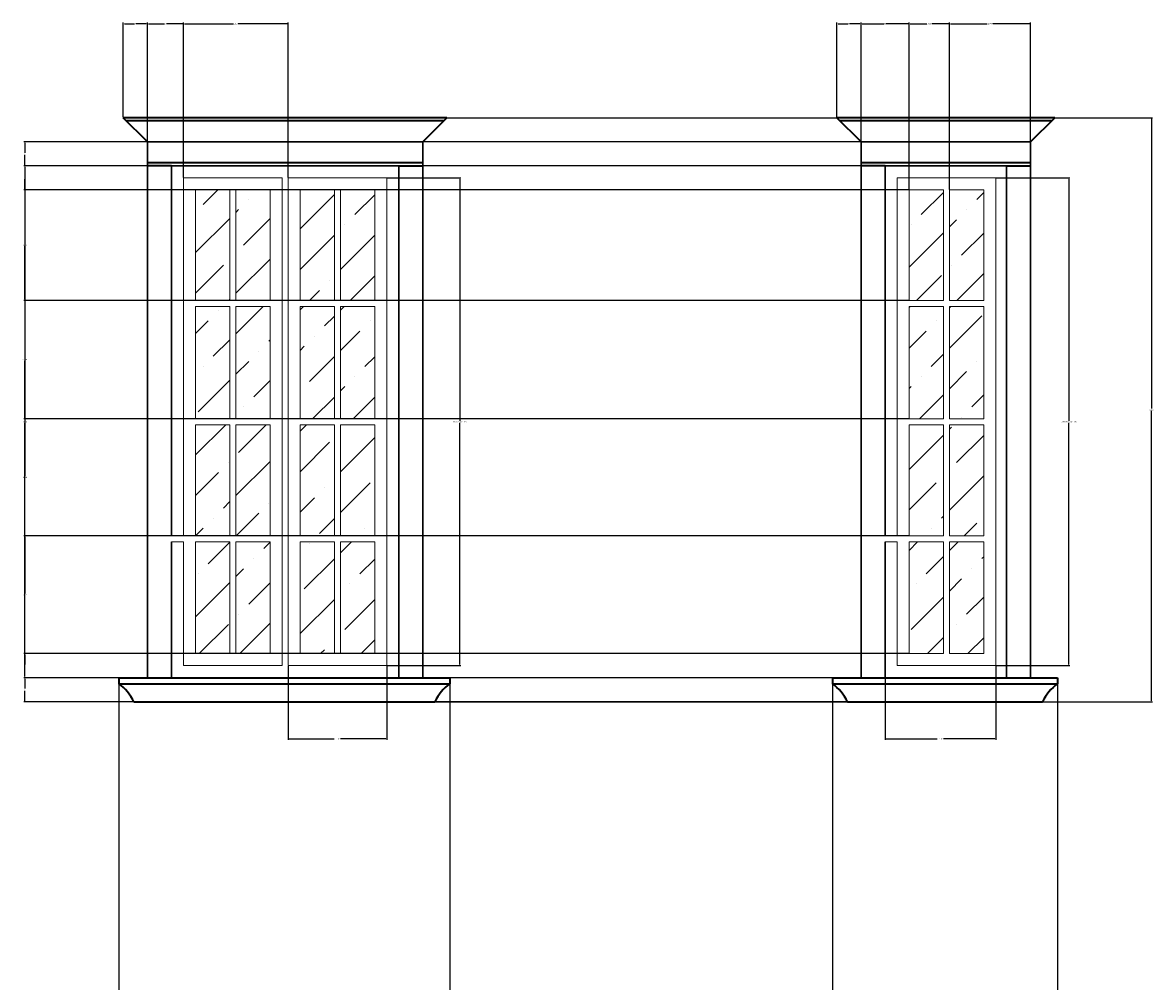
# Model space of a CAD drawing. Units: inches. Extents: x 386 to 708, y 151 to 489.
# Tile 4 of 4: x 520 to 708, y 320 to 479. Entities that reach past the tile are written whole.
import ezdxf

# ---------------------------------------------------------------- set-up
doc = ezdxf.new("R2010")
doc.units = ezdxf.units.IN
doc.header["$MEASUREMENT"] = 0
for name, color, linetype, lineweight in [('A-ANNO-DIMS', 2, 'Continuous', 18), ('A-GLAZ-FRAM', 4, 'Continuous', 30), ('A-GLAZ-PATT', 252, 'Continuous', 13), ('A-GLAZ-SASH', 4, 'Continuous', 18), ('A-GLAZ-SILL', 7, 'Continuous', 35), ('A-GLAZ-TRIM', 7, 'Continuous', 35)]:
    doc.layers.add(name, color=color, linetype=linetype, lineweight=lineweight)
doc.styles.get("Standard").update_dxf_attribs({"font": 'arial.ttf'})
doc.dimstyles.get("Standard").update_dxf_attribs({"dimtxt": 0.18, "dimasz": 0.18, "dimexe": 0.18, "dimexo": 0.0625, "dimgap": 0.09, "dimtad": 0, "dimtih": 1, "dimtoh": 1, "dimdec": 4, "dimzin": 0, "dimdsep": 46, "dimtxsty": 'Standard', "dimcen": 0.09, "dimadec": 0, "dimazin": 0, "dimtfac": 1, "dimtdec": 4, "dimtofl": 0, "dimtmove": 0, "dimatfit": 3, "dimfxl": 1, "dimtolj": 1, "dimtzin": 0, "dimarcsym": 0})

# ---------------------------------------------------------------- blocks, each defined once
blk = doc.blocks.new('WIN-SASH-2X4-L')
for p, q in [((9.69, 60.63), (9.69, 78.96)), ((10.69, 60.63), (10.69, 78.96)), ((4, 60.63), (9.69, 60.63)), ((10.69, 60.63), (16.38, 60.63)), ((4, 59.63), (9.69, 59.63)), ((9.69, 40.98), (9.69, 59.63)), ((10.69, 59.63), (16.38, 59.63)), ((10.69, 40.98), (10.69, 59.63)), ((4, 40.98), (9.69, 40.98)), ((4, 39.98), (9.69, 39.98)), ((9.69, 21.54), (9.69, 39.98)), ((10.69, 40.98), (16.38, 40.98)), ((10.69, 39.98), (16.38, 39.98)), ((10.69, 21.54), (10.69, 39.98)), ((0, 21.54), (2, 21.54)), ((4, 21.54), (9.69, 21.54)), ((10.69, 21.54), (16.38, 21.54)), ((0, 20.54), (2, 20.54)), ((4, 20.54), (9.69, 20.54)), ((9.69, 2), (9.69, 20.54)), ((10.69, 2), (10.69, 20.54)), ((10.69, 20.54), (16.38, 20.54))]:
    blk.add_line(p, q)
for points in [[(2, 20.54), (2, 0), (18.38, 0), (18.38, 80.96), (2, 80.96), (2, 21.54)], [(9.69, 78.96), (4, 78.96), (4, 60.63)], [(16.38, 60.63), (16.38, 78.96), (10.69, 78.96)], [(4, 59.63), (4, 40.98)], [(16.38, 40.98), (16.38, 59.63)], [(4, 39.98), (4, 21.54)], [(16.38, 21.54), (16.38, 39.98)], [(4, 20.54), (4, 2), (9.69, 2)], [(10.69, 2), (16.38, 2), (16.38, 20.54)]]:
    blk.add_lwpolyline(points)
blk = doc.blocks.new('WIN-SASH-2X4-R')
for p, q in [((7.69, 60.63), (7.69, 78.96)), ((8.69, 60.63), (8.69, 78.96)), ((2, 60.63), (7.69, 60.63)), ((8.69, 60.63), (14.38, 60.63)), ((2, 59.63), (7.69, 59.63)), ((7.69, 40.98), (7.69, 59.63)), ((8.69, 40.98), (8.69, 59.63)), ((8.69, 59.63), (14.38, 59.63)), ((2, 40.98), (7.69, 40.98)), ((2, 39.98), (7.69, 39.98)), ((7.69, 21.54), (7.69, 39.98)), ((8.69, 40.98), (14.38, 40.98)), ((8.69, 21.54), (8.69, 39.98)), ((8.69, 39.98), (14.38, 39.98)), ((2, 21.54), (7.69, 21.54)), ((8.69, 21.54), (14.38, 21.54)), ((2, 20.54), (7.69, 20.54)), ((7.69, 2), (7.69, 20.54)), ((8.69, 2), (8.69, 20.54)), ((8.69, 20.54), (14.38, 20.54))]:
    blk.add_line(p, q)
blk.add_lwpolyline([(0, 0), (16.38, 0), (16.38, 80.96), (0, 80.96)], close=True)
for points in [[(7.69, 78.96), (2, 78.96), (2, 60.63)], [(14.38, 60.63), (14.38, 78.96), (8.69, 78.96)], [(2, 59.63), (2, 40.98)], [(14.38, 40.98), (14.38, 59.63)], [(2, 39.98), (2, 21.54)], [(14.38, 21.54), (14.38, 39.98)], [(2, 20.54), (2, 2), (7.69, 2)], [(8.69, 2), (14.38, 2), (14.38, 20.54)]]:
    blk.add_lwpolyline(points)
blk = doc.blocks.new('WIN-SILL-DOUBLE')
for p, q in [((0, 4), (54.98, 4)), ((0, 4), (0, 3)), ((54.98, 4), (54.98, 3)), ((0, 3), (54.98, 3)), ((2.49, 0), (52.48, 0))]:
    blk.add_line(p, q)
blk.add_lwpolyline([(4.75, 0), (50.49, 0)])
for centre, start, end in [((-4.74, -3.48), 25.6893, 53.8074), ((59.72, -3.48), 126.1926, 154.3107)]:
    blk.add_arc(centre, 8.03, start, end)
blk = doc.blocks.new('*D8')
at = {"layer": 'A-ANNO-DIMS', "color": 0, "lineweight": -2, "transparency": 16777216}
for p, q in [((681.69, 453.66), (693.95, 453.66)), ((693.77, 453.48), (693.77, 413.36)), ((693.77, 372.88), (693.77, 413)), ((681.69, 372.7), (693.95, 372.7))]:
    blk.add_line(p, q, dxfattribs=at)
at = {"layer": 'A-ANNO-DIMS', "color": 0, "transparency": 16777216}
for points in [[(693.74, 453.48), (693.8, 453.48), (693.77, 453.66)], [(693.74, 372.88), (693.8, 372.88), (693.77, 372.7)]]:
    blk.add_solid(points, dxfattribs=at)
at = {"layer": 'Defpoints', "color": 0, "transparency": 16777216}
for p in [(681.63, 453.66), (693.77, 453.66), (681.63, 372.7)]:
    blk.add_point(p, dxfattribs=at)
at = {"layer": 'A-ANNO-DIMS', "color": 0, "transparency": 16777216, "insert": (693.77, 413.18), "char_height": 0.18, "attachment_point": 5}
blk.add_mtext('\\A1;NARROW SASH 81 TYP.', dxfattribs=at)
blk = doc.blocks.new('*D9')
at = {"layer": 'A-ANNO-DIMS', "color": 0, "lineweight": -2, "transparency": 16777216}
for p, q in [((663.25, 372.64), (663.25, 360.38)), ((681.63, 372.64), (681.63, 360.38)), ((663.43, 360.56), (671.92, 360.56)), ((681.45, 360.56), (672.96, 360.56))]:
    blk.add_line(p, q, dxfattribs=at)
at = {"layer": 'A-ANNO-DIMS', "color": 0, "transparency": 16777216}
for points in [[(663.43, 360.59), (663.43, 360.53), (663.25, 360.56)], [(681.45, 360.59), (681.45, 360.53), (681.63, 360.56)]]:
    blk.add_solid(points, dxfattribs=at)
at = {"layer": 'Defpoints', "color": 0, "transparency": 16777216}
for p in [(663.25, 372.7), (681.63, 372.7), (681.63, 360.56)]:
    blk.add_point(p, dxfattribs=at)
at = {"layer": 'A-ANNO-DIMS', "color": 0, "transparency": 16777216, "insert": (672.44, 360.56), "char_height": 0.18, "attachment_point": 5}
blk.add_mtext('\\A1;18 TYP.', dxfattribs=at)
blk = doc.blocks.new('*D10')
at = {"layer": 'A-ANNO-DIMS', "color": 0, "lineweight": -2, "transparency": 16777216}
for p, q in [((580.55, 453.66), (592.81, 453.66)), ((592.63, 453.48), (592.63, 413.36)), ((592.63, 372.88), (592.63, 413)), ((580.55, 372.7), (592.81, 372.7))]:
    blk.add_line(p, q, dxfattribs=at)
at = {"layer": 'A-ANNO-DIMS', "color": 0, "transparency": 16777216}
for points in [[(592.6, 453.48), (592.66, 453.48), (592.63, 453.66)], [(592.6, 372.88), (592.66, 372.88), (592.63, 372.7)]]:
    blk.add_solid(points, dxfattribs=at)
at = {"layer": 'Defpoints', "color": 0, "transparency": 16777216}
for p in [(580.49, 453.66), (592.63, 453.66), (580.49, 372.7)]:
    blk.add_point(p, dxfattribs=at)
at = {"layer": 'A-ANNO-DIMS', "color": 0, "transparency": 16777216, "insert": (592.63, 413.18), "char_height": 0.18, "attachment_point": 5}
blk.add_mtext('\\A1;RIGHT SASH 81 TYP.', dxfattribs=at)
blk = doc.blocks.new('*D11')
at = {"layer": 'A-ANNO-DIMS', "color": 0, "lineweight": -2, "transparency": 16777216}
for p, q in [((564.11, 372.64), (564.11, 360.38)), ((580.49, 372.64), (580.49, 360.38)), ((564.29, 360.56), (571.78, 360.56)), ((580.31, 360.56), (572.82, 360.56))]:
    blk.add_line(p, q, dxfattribs=at)
at = {"layer": 'A-ANNO-DIMS', "color": 0, "transparency": 16777216}
for points in [[(564.29, 360.59), (564.29, 360.53), (564.11, 360.56)], [(580.31, 360.59), (580.31, 360.53), (580.49, 360.56)]]:
    blk.add_solid(points, dxfattribs=at)
at = {"layer": 'Defpoints', "color": 0, "transparency": 16777216}
for p in [(564.11, 372.7), (580.49, 372.7), (580.49, 360.56)]:
    blk.add_point(p, dxfattribs=at)
at = {"layer": 'A-ANNO-DIMS', "color": 0, "transparency": 16777216, "insert": (572.3, 360.56), "char_height": 0.18, "attachment_point": 5}
blk.add_mtext('\\A1;16 TYP.', dxfattribs=at)
blk = doc.blocks.new('*D45')
at = {"layer": 'A-ANNO-DIMS', "color": 0, "lineweight": -2, "transparency": 16777216}
for p, q in [((590.55, 463.66), (707.68, 463.66)), ((707.5, 463.48), (707.5, 415.36)), ((707.5, 366.88), (707.5, 415)), ((588.54, 366.7), (707.68, 366.7))]:
    blk.add_line(p, q, dxfattribs=at)
at = {"layer": 'A-ANNO-DIMS', "color": 0, "transparency": 16777216}
for points in [[(707.47, 463.48), (707.53, 463.48), (707.5, 463.66)], [(707.47, 366.88), (707.53, 366.88), (707.5, 366.7)]]:
    blk.add_solid(points, dxfattribs=at)
at = {"layer": 'Defpoints', "color": 0, "transparency": 16777216}
for p in [(590.49, 463.66), (707.5, 463.66), (588.47, 366.7)]:
    blk.add_point(p, dxfattribs=at)
at = {"layer": 'A-ANNO-DIMS', "color": 0, "transparency": 16777216, "insert": (707.5, 415.18), "char_height": 0.18, "attachment_point": 5}
blk.add_mtext('\\A1;96.96', dxfattribs=at)
blk = doc.blocks.new('*D46')
at = {"layer": 'A-ANNO-DIMS', "color": 0, "lineweight": -2, "transparency": 16777216}
for p, q in [((540.67, 455.66), (520.21, 455.66)), ((520.39, 455.48), (520.39, 413.36)), ((520.39, 370.88), (520.39, 413)), ((535.93, 370.7), (520.21, 370.7))]:
    blk.add_line(p, q, dxfattribs=at)
at = {"layer": 'A-ANNO-DIMS', "color": 0, "transparency": 16777216}
for points in [[(520.36, 455.48), (520.42, 455.48), (520.39, 455.66)], [(520.36, 370.88), (520.42, 370.88), (520.39, 370.7)]]:
    blk.add_solid(points, dxfattribs=at)
at = {"layer": 'Defpoints', "color": 0, "transparency": 16777216}
for p in [(520.39, 455.66), (540.74, 455.66), (535.99, 370.7)]:
    blk.add_point(p, dxfattribs=at)
at = {"layer": 'A-ANNO-DIMS', "color": 0, "transparency": 16777216, "insert": (520.39, 413.18), "char_height": 0.18, "attachment_point": 5}
blk.add_mtext('\\A1;84.96', dxfattribs=at)
blk = doc.blocks.new('*D47')
at = {"layer": 'A-ANNO-DIMS', "color": 0, "lineweight": -2, "transparency": 16777216}
for p, q in [((535.99, 370.64), (535.99, 151.47)), ((590.97, 370.64), (590.97, 151.47)), ((536.17, 151.65), (563.09, 151.65)), ((590.79, 151.65), (563.87, 151.65))]:
    blk.add_line(p, q, dxfattribs=at)
at = {"layer": 'A-ANNO-DIMS', "color": 0, "transparency": 16777216}
for points in [[(536.17, 151.68), (536.17, 151.62), (535.99, 151.65)], [(590.79, 151.68), (590.79, 151.62), (590.97, 151.65)]]:
    blk.add_solid(points, dxfattribs=at)
at = {"layer": 'Defpoints', "color": 0, "transparency": 16777216}
for p in [(535.99, 370.7), (590.97, 370.7), (590.97, 151.65)]:
    blk.add_point(p, dxfattribs=at)
at = {"layer": 'A-ANNO-DIMS', "color": 0, "transparency": 16777216, "insert": (563.48, 151.65), "char_height": 0.18, "attachment_point": 5}
blk.add_mtext('\\A1;54.98', dxfattribs=at)
blk = doc.blocks.new('*D48')
at = {"layer": 'A-ANNO-DIMS', "color": 0, "lineweight": -2, "transparency": 16777216}
for p, q in [((536.74, 463.72), (536.74, 479.44)), ((536.92, 479.26), (538.58, 479.26)), ((540.56, 479.26), (538.89, 479.26)), ((540.74, 459.72), (540.74, 479.44))]:
    blk.add_line(p, q, dxfattribs=at)
at = {"layer": 'A-ANNO-DIMS', "color": 0, "transparency": 16777216}
for points in [[(536.92, 479.29), (536.92, 479.23), (536.74, 479.26)], [(540.56, 479.29), (540.56, 479.23), (540.74, 479.26)]]:
    blk.add_solid(points, dxfattribs=at)
at = {"layer": 'Defpoints', "color": 0, "transparency": 16777216}
for p in [(540.74, 479.26), (536.74, 463.66), (540.74, 459.66)]:
    blk.add_point(p, dxfattribs=at)
at = {"layer": 'A-ANNO-DIMS', "color": 0, "transparency": 16777216, "insert": (538.74, 479.26), "char_height": 0.18, "attachment_point": 5}
blk.add_mtext('\\A1;4', dxfattribs=at)
blk = doc.blocks.new('*D49')
at = {"layer": 'A-ANNO-DIMS', "color": 0, "lineweight": -2, "transparency": 16777216}
for p, q in [((540.74, 459.72), (540.74, 479.44)), ((540.92, 479.26), (543.59, 479.26)), ((546.56, 479.26), (543.89, 479.26)), ((546.74, 453.72), (546.74, 479.44))]:
    blk.add_line(p, q, dxfattribs=at)
at = {"layer": 'A-ANNO-DIMS', "color": 0, "transparency": 16777216}
for points in [[(540.92, 479.29), (540.92, 479.23), (540.74, 479.26)], [(546.56, 479.29), (546.56, 479.23), (546.74, 479.26)]]:
    blk.add_solid(points, dxfattribs=at)
at = {"layer": 'Defpoints', "color": 0, "transparency": 16777216}
for p in [(546.74, 479.26), (540.74, 459.66), (546.74, 453.66)]:
    blk.add_point(p, dxfattribs=at)
at = {"layer": 'A-ANNO-DIMS', "color": 0, "transparency": 16777216, "insert": (543.74, 479.26), "char_height": 0.18, "attachment_point": 5}
blk.add_mtext('\\A1;6', dxfattribs=at)
blk = doc.blocks.new('*D50')
at = {"layer": 'A-ANNO-DIMS', "color": 0, "lineweight": -2, "transparency": 16777216}
for p, q in [((546.74, 453.72), (546.74, 479.44)), ((546.92, 479.26), (555.04, 479.26)), ((563.93, 479.26), (555.81, 479.26)), ((564.11, 453.72), (564.11, 479.44))]:
    blk.add_line(p, q, dxfattribs=at)
at = {"layer": 'A-ANNO-DIMS', "color": 0, "transparency": 16777216}
for points in [[(546.92, 479.29), (546.92, 479.23), (546.74, 479.26)], [(563.93, 479.29), (563.93, 479.23), (564.11, 479.26)]]:
    blk.add_solid(points, dxfattribs=at)
at = {"layer": 'Defpoints', "color": 0, "transparency": 16777216}
for p in [(564.11, 479.26), (546.74, 453.66), (564.11, 453.66)]:
    blk.add_point(p, dxfattribs=at)
at = {"layer": 'A-ANNO-DIMS', "color": 0, "transparency": 16777216, "insert": (555.42, 479.26), "char_height": 0.18, "attachment_point": 5}
blk.add_mtext('\\A1;17.37', dxfattribs=at)
blk = doc.blocks.new('*D51')
at = {"layer": 'A-ANNO-DIMS', "color": 0, "lineweight": -2, "transparency": 16777216}
for p, q in [((654.5, 370.64), (654.5, 151.47)), ((691.9, 370.64), (691.9, 151.47)), ((654.68, 151.65), (672.88, 151.65)), ((691.72, 151.65), (673.53, 151.65))]:
    blk.add_line(p, q, dxfattribs=at)
at = {"layer": 'A-ANNO-DIMS', "color": 0, "transparency": 16777216}
for points in [[(654.68, 151.68), (654.68, 151.62), (654.5, 151.65)], [(691.72, 151.68), (691.72, 151.62), (691.9, 151.65)]]:
    blk.add_solid(points, dxfattribs=at)
at = {"layer": 'Defpoints', "color": 0, "transparency": 16777216}
for p in [(654.5, 370.7), (691.9, 370.7), (691.9, 151.65)]:
    blk.add_point(p, dxfattribs=at)
at = {"layer": 'A-ANNO-DIMS', "color": 0, "transparency": 16777216, "insert": (673.2, 151.65), "char_height": 0.18, "attachment_point": 5}
blk.add_mtext('\\A1;37.4', dxfattribs=at)
blk = doc.blocks.new('*D52')
at = {"layer": 'A-ANNO-DIMS', "color": 0, "lineweight": -2, "transparency": 16777216}
for p, q in [((691.48, 463.66), (707.68, 463.66)), ((707.5, 463.48), (707.5, 415.36)), ((707.5, 366.88), (707.5, 415)), ((689.47, 366.7), (707.68, 366.7))]:
    blk.add_line(p, q, dxfattribs=at)
at = {"layer": 'A-ANNO-DIMS', "color": 0, "transparency": 16777216}
for points in [[(707.47, 463.48), (707.53, 463.48), (707.5, 463.66)], [(707.47, 366.88), (707.53, 366.88), (707.5, 366.7)]]:
    blk.add_solid(points, dxfattribs=at)
at = {"layer": 'Defpoints', "color": 0, "transparency": 16777216}
for p in [(691.42, 463.66), (707.5, 463.66), (689.41, 366.7)]:
    blk.add_point(p, dxfattribs=at)
at = {"layer": 'A-ANNO-DIMS', "color": 0, "transparency": 16777216, "insert": (707.5, 415.18), "char_height": 0.18, "attachment_point": 5}
blk.add_mtext('\\A1;96.96', dxfattribs=at)
blk = doc.blocks.new('*D53')
at = {"layer": 'A-ANNO-DIMS', "color": 0, "lineweight": -2, "transparency": 16777216}
for p, q in [((655.25, 463.72), (655.25, 479.44)), ((655.43, 479.26), (657.1, 479.26)), ((659.07, 479.26), (657.4, 479.26)), ((659.25, 459.72), (659.25, 479.44))]:
    blk.add_line(p, q, dxfattribs=at)
at = {"layer": 'A-ANNO-DIMS', "color": 0, "transparency": 16777216}
for points in [[(655.43, 479.29), (655.43, 479.23), (655.25, 479.26)], [(659.07, 479.29), (659.07, 479.23), (659.25, 479.26)]]:
    blk.add_solid(points, dxfattribs=at)
at = {"layer": 'Defpoints', "color": 0, "transparency": 16777216}
for p in [(659.25, 479.26), (655.25, 463.66), (659.25, 459.66)]:
    blk.add_point(p, dxfattribs=at)
at = {"layer": 'A-ANNO-DIMS', "color": 0, "transparency": 16777216, "insert": (657.25, 479.26), "char_height": 0.18, "attachment_point": 5}
blk.add_mtext('\\A1;4', dxfattribs=at)
blk = doc.blocks.new('*D54')
at = {"layer": 'A-ANNO-DIMS', "color": 0, "lineweight": -2, "transparency": 16777216}
for p, q in [((659.25, 459.72), (659.25, 479.44)), ((659.43, 479.26), (663.1, 479.26)), ((667.07, 479.26), (663.4, 479.26)), ((667.25, 451.72), (667.25, 479.44))]:
    blk.add_line(p, q, dxfattribs=at)
at = {"layer": 'A-ANNO-DIMS', "color": 0, "transparency": 16777216}
for points in [[(659.43, 479.29), (659.43, 479.23), (659.25, 479.26)], [(667.07, 479.29), (667.07, 479.23), (667.25, 479.26)]]:
    blk.add_solid(points, dxfattribs=at)
at = {"layer": 'Defpoints', "color": 0, "transparency": 16777216}
for p in [(667.25, 479.26), (659.25, 459.66), (667.25, 451.66)]:
    blk.add_point(p, dxfattribs=at)
at = {"layer": 'A-ANNO-DIMS', "color": 0, "transparency": 16777216, "insert": (663.25, 479.26), "char_height": 0.18, "attachment_point": 5}
blk.add_mtext('\\A1;8', dxfattribs=at)
blk = doc.blocks.new('*D55')
at = {"layer": 'A-ANNO-DIMS', "color": 0, "lineweight": -2, "transparency": 16777216}
for p, q in [((667.25, 451.72), (667.25, 479.44)), ((667.43, 479.26), (670.2, 479.26)), ((673.76, 479.26), (670.99, 479.26)), ((673.94, 451.72), (673.94, 479.44))]:
    blk.add_line(p, q, dxfattribs=at)
at = {"layer": 'A-ANNO-DIMS', "color": 0, "transparency": 16777216}
for points in [[(667.43, 479.29), (667.43, 479.23), (667.25, 479.26)], [(673.76, 479.29), (673.76, 479.23), (673.94, 479.26)]]:
    blk.add_solid(points, dxfattribs=at)
at = {"layer": 'Defpoints', "color": 0, "transparency": 16777216}
for p in [(673.94, 479.26), (667.25, 451.66), (673.94, 451.66)]:
    blk.add_point(p, dxfattribs=at)
at = {"layer": 'A-ANNO-DIMS', "color": 0, "transparency": 16777216, "insert": (670.59, 479.26), "char_height": 0.18, "attachment_point": 5}
blk.add_mtext('\\A1;6.689', dxfattribs=at)
blk = doc.blocks.new('*D56')
at = {"layer": 'A-ANNO-DIMS', "color": 0, "lineweight": -2, "transparency": 16777216}
for p, q in [((673.94, 451.72), (673.94, 479.44)), ((674.12, 479.26), (680.22, 479.26)), ((687.24, 479.26), (681.13, 479.26)), ((687.42, 459.72), (687.42, 479.44))]:
    blk.add_line(p, q, dxfattribs=at)
at = {"layer": 'A-ANNO-DIMS', "color": 0, "transparency": 16777216}
for points in [[(674.12, 479.29), (674.12, 479.23), (673.94, 479.26)], [(687.24, 479.29), (687.24, 479.23), (687.42, 479.26)]]:
    blk.add_solid(points, dxfattribs=at)
at = {"layer": 'Defpoints', "color": 0, "transparency": 16777216}
for p in [(687.42, 479.26), (687.42, 459.66), (673.94, 451.66)]:
    blk.add_point(p, dxfattribs=at)
at = {"layer": 'A-ANNO-DIMS', "color": 0, "transparency": 16777216, "insert": (680.68, 479.26), "char_height": 0.18, "attachment_point": 5}
blk.add_mtext('\\A1;13.478', dxfattribs=at)
blk = doc.blocks.new('*D57')
at = {"layer": 'A-ANNO-DIMS', "color": 0, "lineweight": -2, "transparency": 16777216}
for p, q in [((654.44094, 370.702039), (520.210553, 370.702039)), ((520.390553, 370.522039), (520.390553, 368.882039)), ((520.390553, 366.882039), (520.390553, 368.522039)), ((656.935867, 366.702039), (520.210553, 366.702039))]:
    blk.add_line(p, q, dxfattribs=at)
at = {"layer": 'A-ANNO-DIMS', "color": 0, "transparency": 16777216}
for points in [[(520.360553, 370.522039), (520.420553, 370.522039), (520.390553, 370.702039)], [(520.360553, 366.882039), (520.420553, 366.882039), (520.390553, 366.702039)]]:
    blk.add_solid(points, dxfattribs=at)
at = {"layer": 'Defpoints', "color": 0, "transparency": 16777216}
for p in [(520.390553, 370.702039), (654.50344, 370.702039), (656.998367, 366.702039)]:
    blk.add_point(p, dxfattribs=at)
at = {"layer": 'A-ANNO-DIMS', "color": 0, "transparency": 16777216, "insert": (520.390553, 368.702039), "char_height": 0.18, "attachment_point": 5}
blk.add_mtext('\\A1;4', dxfattribs=at)
blk = doc.blocks.new('*D58')
at = {"layer": 'A-ANNO-DIMS', "color": 0, "lineweight": -2, "transparency": 16777216}
for p, q in [((667.187175, 374.702039), (520.210553, 374.702039)), ((520.390553, 374.522039), (520.390553, 372.882039)), ((520.390553, 370.882039), (520.390553, 372.522039)), ((654.44094, 370.702039), (520.210553, 370.702039))]:
    blk.add_line(p, q, dxfattribs=at)
at = {"layer": 'A-ANNO-DIMS', "color": 0, "transparency": 16777216}
for points in [[(520.360553, 374.522039), (520.420553, 374.522039), (520.390553, 374.702039)], [(520.360553, 370.882039), (520.420553, 370.882039), (520.390553, 370.702039)]]:
    blk.add_solid(points, dxfattribs=at)
at = {"layer": 'Defpoints', "color": 0, "transparency": 16777216}
for p in [(520.390553, 374.702039), (667.249675, 374.702039), (654.50344, 370.702039)]:
    blk.add_point(p, dxfattribs=at)
at = {"layer": 'A-ANNO-DIMS', "color": 0, "transparency": 16777216, "insert": (520.390553, 372.702039), "char_height": 0.18, "attachment_point": 5}
blk.add_mtext('\\A1;4', dxfattribs=at)
blk = doc.blocks.new('*D59')
at = {"layer": 'A-ANNO-DIMS', "color": 0, "lineweight": -2, "transparency": 16777216}
for p, q in [((667.19, 394.24), (520.21, 394.24)), ((520.39, 394.06), (520.39, 384.65)), ((520.39, 374.88), (520.39, 384.29)), ((667.19, 374.7), (520.21, 374.7))]:
    blk.add_line(p, q, dxfattribs=at)
at = {"layer": 'A-ANNO-DIMS', "color": 0, "transparency": 16777216}
for points in [[(520.36, 394.06), (520.42, 394.06), (520.39, 394.24)], [(520.36, 374.88), (520.42, 374.88), (520.39, 374.7)]]:
    blk.add_solid(points, dxfattribs=at)
at = {"layer": 'Defpoints', "color": 0, "transparency": 16777216}
for p in [(520.39, 394.24), (667.25, 394.24), (667.25, 374.7)]:
    blk.add_point(p, dxfattribs=at)
at = {"layer": 'A-ANNO-DIMS', "color": 0, "transparency": 16777216, "insert": (520.39, 384.47), "char_height": 0.18, "attachment_point": 5}
blk.add_mtext('\\A1;19.537', dxfattribs=at)
blk = doc.blocks.new('*D60')
at = {"layer": 'A-ANNO-DIMS', "color": 0, "lineweight": -2, "transparency": 16777216}
for p, q in [((667.19, 413.68), (520.21, 413.68)), ((520.39, 413.5), (520.39, 404.14)), ((520.39, 394.42), (520.39, 403.78)), ((667.19, 394.24), (520.21, 394.24))]:
    blk.add_line(p, q, dxfattribs=at)
at = {"layer": 'A-ANNO-DIMS', "color": 0, "transparency": 16777216}
for points in [[(520.36, 413.5), (520.42, 413.5), (520.39, 413.68)], [(520.36, 394.42), (520.42, 394.42), (520.39, 394.24)]]:
    blk.add_solid(points, dxfattribs=at)
at = {"layer": 'Defpoints', "color": 0, "transparency": 16777216}
for p in [(520.39, 413.68), (667.25, 413.68), (667.25, 394.24)]:
    blk.add_point(p, dxfattribs=at)
at = {"layer": 'A-ANNO-DIMS', "color": 0, "transparency": 16777216, "insert": (520.39, 403.96), "char_height": 0.18, "attachment_point": 5}
blk.add_mtext('\\A1;19.44', dxfattribs=at)
blk = doc.blocks.new('*D61')
at = {"layer": 'A-ANNO-DIMS', "color": 0, "lineweight": -2, "transparency": 16777216}
for p, q in [((667.19, 433.33), (520.21, 433.33)), ((520.39, 433.15), (520.39, 423.69)), ((520.39, 413.86), (520.39, 423.32)), ((667.19, 413.68), (520.21, 413.68))]:
    blk.add_line(p, q, dxfattribs=at)
at = {"layer": 'A-ANNO-DIMS', "color": 0, "transparency": 16777216}
for points in [[(520.36, 433.15), (520.42, 433.15), (520.39, 433.33)], [(520.36, 413.86), (520.42, 413.86), (520.39, 413.68)]]:
    blk.add_solid(points, dxfattribs=at)
at = {"layer": 'Defpoints', "color": 0, "transparency": 16777216}
for p in [(520.39, 433.33), (667.25, 433.33), (667.25, 413.68)]:
    blk.add_point(p, dxfattribs=at)
at = {"layer": 'A-ANNO-DIMS', "color": 0, "transparency": 16777216, "insert": (520.39, 423.5), "char_height": 0.18, "attachment_point": 5}
blk.add_mtext('\\A1;19.648', dxfattribs=at)
blk = doc.blocks.new('*D62')
at = {"layer": 'A-ANNO-DIMS', "color": 0, "lineweight": -2, "transparency": 16777216}
for p, q in [((667.19, 451.66), (520.21, 451.66)), ((520.39, 451.48), (520.39, 442.67)), ((520.39, 433.51), (520.39, 442.31)), ((667.19, 433.33), (520.21, 433.33))]:
    blk.add_line(p, q, dxfattribs=at)
at = {"layer": 'A-ANNO-DIMS', "color": 0, "transparency": 16777216}
for points in [[(520.36, 451.48), (520.42, 451.48), (520.39, 451.66)], [(520.36, 433.51), (520.42, 433.51), (520.39, 433.33)]]:
    blk.add_solid(points, dxfattribs=at)
at = {"layer": 'Defpoints', "color": 0, "transparency": 16777216}
for p in [(520.39, 451.66), (667.25, 451.66), (667.25, 433.33)]:
    blk.add_point(p, dxfattribs=at)
at = {"layer": 'A-ANNO-DIMS', "color": 0, "transparency": 16777216, "insert": (520.39, 442.49), "char_height": 0.18, "attachment_point": 5}
blk.add_mtext('\\A1;18.33', dxfattribs=at)
blk = doc.blocks.new('*D63')
at = {"layer": 'A-ANNO-DIMS', "color": 0, "lineweight": -2, "transparency": 16777216}
for p, q in [((659.187175, 455.657677), (520.210553, 455.657677)), ((520.390553, 455.477677), (520.390553, 453.837677)), ((520.390553, 451.837677), (520.390553, 453.477677)), ((667.187175, 451.657677), (520.210553, 451.657677))]:
    blk.add_line(p, q, dxfattribs=at)
at = {"layer": 'A-ANNO-DIMS', "color": 0, "transparency": 16777216}
for points in [[(520.360553, 455.477677), (520.420553, 455.477677), (520.390553, 455.657677)], [(520.360553, 451.837677), (520.420553, 451.837677), (520.390553, 451.657677)]]:
    blk.add_solid(points, dxfattribs=at)
at = {"layer": 'Defpoints', "color": 0, "transparency": 16777216}
for p in [(520.390553, 455.657677), (659.249675, 455.657677), (667.249675, 451.657677)]:
    blk.add_point(p, dxfattribs=at)
at = {"layer": 'A-ANNO-DIMS', "color": 0, "transparency": 16777216, "insert": (520.390553, 453.657677), "char_height": 0.18, "attachment_point": 5}
blk.add_mtext('\\A1;4', dxfattribs=at)
blk = doc.blocks.new('*D64')
at = {"layer": 'A-ANNO-DIMS', "color": 0, "lineweight": -2, "transparency": 16777216}
for p, q in [((659.187175, 459.657677), (520.210553, 459.657677)), ((520.390553, 459.477677), (520.390553, 457.837677)), ((520.390553, 455.837677), (520.390553, 457.477677)), ((659.187175, 455.657677), (520.210553, 455.657677))]:
    blk.add_line(p, q, dxfattribs=at)
at = {"layer": 'A-ANNO-DIMS', "color": 0, "transparency": 16777216}
for points in [[(520.360553, 459.477677), (520.420553, 459.477677), (520.390553, 459.657677)], [(520.360553, 455.837677), (520.420553, 455.837677), (520.390553, 455.657677)]]:
    blk.add_solid(points, dxfattribs=at)
at = {"layer": 'Defpoints', "color": 0, "transparency": 16777216}
for p in [(520.390553, 459.657677), (659.249675, 459.657677), (659.249675, 455.657677)]:
    blk.add_point(p, dxfattribs=at)
at = {"layer": 'A-ANNO-DIMS', "color": 0, "transparency": 16777216, "insert": (520.390553, 457.657677), "char_height": 0.18, "attachment_point": 5}
blk.add_mtext('\\A1;4', dxfattribs=at)

msp = doc.modelspace()

# ---------------------------------------------------------------- hatches: boundary and pattern name
at = {"layer": 'A-GLAZ-PATT'}
h = msp.add_hatch(dxfattribs=at)
h.set_pattern_fill('ANSI36', color=256, scale=38)
h.paths.add_polyline_path([(569.9858, 191.2056), (557.2368, 191.2056), (557.2368, 173.751), (569.9858, 173.751)])
h.paths.add_polyline_path([(556.7368, 191.2056), (547.2368, 191.2056), (547.2368, 173.751), (556.7368, 173.751)])
h.paths.add_polyline_path([(556.7368, 206.7626), (547.2368, 206.7626), (547.2368, 191.7056), (556.7368, 191.7056)])
h.paths.add_polyline_path([(569.9858, 206.7626), (557.2368, 206.7626), (557.2368, 191.7056), (569.9858, 191.7056)])
h.paths.add_polyline_path([(579.9858, 206.7626), (570.4858, 206.7626), (570.4858, 191.7056), (579.9858, 191.7056)])
h.paths.add_polyline_path([(579.9858, 191.2056), (570.4858, 191.2056), (570.4858, 173.751), (579.9858, 173.751)])
h.paths.add_polyline_path([(579.9858, 225.0121), (570.4858, 225.0121), (570.4858, 207.2626), (579.9858, 207.2626)])
h.paths.add_polyline_path([(569.9858, 225.0121), (557.2368, 225.0121), (557.2368, 207.2626), (569.9858, 207.2626)])
h.paths.add_polyline_path([(556.7368, 225.0121), (547.2368, 225.0121), (547.2368, 207.2626), (556.7368, 207.2626)])
h.paths.add_polyline_path([(556.7368, 241.1674), (547.2368, 241.1674), (547.2368, 225.5121), (556.7368, 225.5121)])
h.paths.add_polyline_path([(569.9858, 241.1674), (557.2368, 241.1674), (557.2368, 225.5121), (569.9858, 225.5121)])
h.paths.add_polyline_path([(579.9858, 241.1674), (570.4858, 241.1674), (570.4858, 225.5121), (579.9858, 225.5121)])
h.paths.add_polyline_path([(579.9858, 256.2066), (570.4858, 256.2066), (570.4858, 241.6674), (579.9858, 241.6674)])
h.paths.add_polyline_path([(569.9858, 256.2066), (557.2368, 256.2066), (557.2368, 241.6674), (569.9858, 241.6674)])
h.paths.add_polyline_path([(556.7368, 256.2066), (547.2368, 256.2066), (547.2368, 241.6674), (556.7368, 241.6674)])
h.paths.add_polyline_path([(570.4676, 256.7066), (579.9782, 256.7066, 0.96991703), (547.2444, 256.7066), (556.755, 256.7066, -0.92973)])
h.paths.add_polyline_path([(557.2564, 256.7066), (569.9662, 256.7066, 0.92441074)], flags=17)
h.paths.add_polyline_path([(578.4858, 393.239), (572.7969, 393.239), (572.7969, 374.702), (578.4858, 374.702)])
h.paths.add_polyline_path([(571.7969, 393.239), (566.1079, 393.239), (566.1079, 374.702), (571.7969, 374.702)])
h.paths.add_polyline_path([(561.1147, 393.239), (555.4258, 393.239), (555.4258, 374.702), (561.1147, 374.702)])
h.paths.add_polyline_path([(554.4258, 393.239), (548.7368, 393.239), (548.7368, 374.702), (554.4258, 374.702)])
h.paths.add_polyline_path([(554.4258, 412.6799), (548.7368, 412.6799), (548.7368, 394.239), (554.4258, 394.239)])
h.paths.add_polyline_path([(561.1147, 412.6799), (555.4258, 412.6799), (555.4258, 394.239), (561.1147, 394.239)])
h.paths.add_polyline_path([(571.7969, 412.6799), (566.1079, 412.6799), (566.1079, 394.239), (571.7969, 394.239)])
h.paths.add_polyline_path([(578.4858, 412.6799), (572.7969, 412.6799), (572.7969, 394.239), (578.4858, 394.239)])
h.paths.add_polyline_path([(578.4858, 432.3276), (572.7969, 432.3276), (572.7969, 413.6799), (578.4858, 413.6799)])
h.paths.add_polyline_path([(571.7969, 432.3276), (566.1079, 432.3276), (566.1079, 413.6799), (571.7969, 413.6799)])
h.paths.add_polyline_path([(561.1147, 432.3276), (555.4258, 432.3276), (555.4258, 413.6799), (561.1147, 413.6799)])
h.paths.add_polyline_path([(554.4258, 432.3276), (548.7368, 432.3276), (548.7368, 413.6799), (554.4258, 413.6799)])
h.paths.add_polyline_path([(554.4258, 451.6577), (548.7368, 451.6577), (548.7368, 433.3276), (554.4258, 433.3276)])
h.paths.add_polyline_path([(561.1147, 451.6577), (555.4258, 451.6577), (555.4258, 433.3276), (561.1147, 433.3276)])
h.paths.add_polyline_path([(571.7969, 451.6577), (566.1079, 451.6577), (566.1079, 433.3276), (571.7969, 433.3276)])
h.paths.add_polyline_path([(578.4858, 451.6577), (572.7969, 451.6577), (572.7969, 433.3276), (578.4858, 433.3276)])
h.paths.add_polyline_path([(672.9386, 451.6577), (667.2497, 451.6577), (667.2497, 433.3276), (672.9386, 433.3276)])
h.paths.add_polyline_path([(679.6276, 451.6577), (673.9386, 451.6577), (673.9386, 433.3276), (679.6276, 433.3276)])
h.paths.add_polyline_path([(679.6276, 432.3276), (673.9386, 432.3276), (673.9386, 413.6799), (679.6276, 413.6799)])
h.paths.add_polyline_path([(672.9386, 432.3276), (667.2497, 432.3276), (667.2497, 413.6799), (672.9386, 413.6799)])
h.paths.add_polyline_path([(672.9386, 412.6799), (667.2497, 412.6799), (667.2497, 394.239), (672.9386, 394.239)])
h.paths.add_polyline_path([(679.6276, 412.6799), (673.9386, 412.6799), (673.9386, 394.239), (679.6276, 394.239)])
h.paths.add_polyline_path([(679.6276, 393.239), (673.9386, 393.239), (673.9386, 374.702), (679.6276, 374.702)])
h.paths.add_polyline_path([(672.9386, 393.239), (667.2497, 393.239), (667.2497, 374.702), (672.9386, 374.702)])

# ---------------------------------------------------------------- linework, layer by layer
at = {"layer": 'A-GLAZ-FRAM'}
for points in [[(586.4858, 370.702), (586.4858, 459.6577), (540.7368, 459.6577)], [(563.5835, 459.6577), (540.7368, 459.6577), (540.7368, 370.702)], [(687.417, 370.702), (687.417, 459.6577), (659.2497, 459.6577)], [(682.0964, 459.6577), (659.2497, 459.6577), (659.2497, 370.702)], [(563.1147, 455.6577), (544.7368, 455.6577), (544.7368, 394.239)], [(544.7368, 393.239), (544.7368, 370.702), (582.4858, 370.702), (582.4858, 455.6577), (564.1079, 455.6577)], [(582.4858, 455.6577), (544.7368, 455.6577)], [(681.6276, 455.6577), (663.2497, 455.6577), (663.2497, 394.239)], [(663.2497, 393.239), (663.2497, 370.702), (683.417, 370.702), (683.417, 455.6577), (682.6208, 455.6577)], [(683.417, 455.6577), (663.2497, 455.6577)]]:
    msp.add_lwpolyline(points, dxfattribs=at)
at = {"layer": 'A-GLAZ-SILL'}
for p, q in [((654.5034, 370.702), (691.9, 370.702)), ((654.5034, 370.702), (654.5034, 369.702)), ((691.9, 370.702), (691.9, 369.702)), ((654.5034, 369.702), (691.9, 369.702)), ((656.9984, 366.702), (689.4051, 366.702))]:
    msp.add_line(p, q, dxfattribs=at)
msp.add_lwpolyline([(659.2497, 366.702), (687.417, 366.702)], dxfattribs=at)
for centre, start, end in [((649.7611, 363.2206), 25.689256, 53.807433), ((696.6424, 363.2206), 126.192567, 154.310744)]:
    msp.add_arc(centre, 8.0311, start, end, dxfattribs=at)
at = {"layer": 'A-GLAZ-TRIM'}
for p, q in [((540.7368, 459.6577), (536.7368, 463.6577)), ((586.4858, 459.6577), (590.4858, 463.6577)), ((659.2497, 459.6577), (655.2497, 463.6577)), ((687.417, 459.6577), (691.417, 463.6577)), ((544.7368, 455.6577), (540.7368, 455.6577)), ((582.4858, 455.6577), (586.4858, 455.6577)), ((663.2497, 455.6577), (659.2497, 455.6577)), ((683.417, 455.6577), (687.417, 455.6577))]:
    msp.add_line(p, q, dxfattribs=at)
for points in [[(590.4858, 463.6577), (536.7368, 463.6577)], [(560.6741, 463.6577), (536.7368, 463.6577)], [(589.9858, 463.1577), (537.2368, 463.1577)], [(561.0139, 463.1577), (537.2368, 463.1577)], [(691.417, 463.6577), (655.2497, 463.6577)], [(679.187, 463.6577), (655.2497, 463.6577)], [(690.917, 463.1577), (655.7497, 463.1577)], [(679.5268, 463.1577), (655.7497, 463.1577)], [(586.4858, 456.1577), (540.7368, 456.1577)], [(687.417, 456.1577), (659.2497, 456.1577)]]:
    msp.add_lwpolyline(points, dxfattribs=at)

# ---------------------------------------------------------------- block references
at = {"layer": 'A-GLAZ-SASH'}
for name, p in [('WIN-SASH-2X4-L', (544.7364, 372.702)), ('WIN-SASH-2X4-R', (564.1083, 372.702)), ('WIN-SASH-2X4-L', (663.2493, 372.702))]:
    msp.add_blockref(name, p, dxfattribs=at)
at = {"layer": 'A-GLAZ-SILL'}
msp.add_blockref('WIN-SILL-DOUBLE', (535.991, 366.702), dxfattribs=at)

# ---------------------------------------------------------------- dimensions: what is measured, and where the dimension line sits
at = {"layer": 'A-ANNO-DIMS'}
for base, p1, p2, override, picture, middle in [((540.7368, 479.2577), (536.7368, 463.6577), (540.7368, 459.6577), {"dimdec": 0, "dimlfac": 1, "dimrnd": 0, "dimzin": 0, "dimdsep": 46, "dimlunit": 2}, '*D48', (538.7368, 479.2577)), ((546.7368, 479.2577), (540.7368, 459.6577), (546.7368, 453.6577), {"dimdec": 0, "dimlfac": 1, "dimrnd": 0, "dimzin": 0, "dimdsep": 46, "dimlunit": 2}, '*D49', (543.7368, 479.2577)), ((564.1079, 479.2577), (546.7368, 453.6577), (564.1079, 453.6577), {"dimdec": 2, "dimlfac": 1, "dimrnd": 0, "dimzin": 0, "dimdsep": 46, "dimlunit": 2}, '*D50', (555.4223, 479.2577)), ((659.2497, 479.2577), (655.2497, 463.6577), (659.2497, 459.6577), {"dimdec": 0, "dimlfac": 1, "dimrnd": 0, "dimzin": 0, "dimdsep": 46, "dimlunit": 2}, '*D53', (657.2497, 479.2577)), ((667.2497, 479.2577), (659.2497, 459.6577), (667.2497, 451.6577), {"dimdec": 0, "dimlfac": 1, "dimrnd": 0, "dimzin": 0, "dimdsep": 46, "dimlunit": 2}, '*D54', (663.2497, 479.2577)), ((673.9386, 479.2577), (667.2497, 451.6577), (673.9386, 451.6577), {"dimdec": 3, "dimlfac": 1, "dimrnd": 0, "dimzin": 0, "dimdsep": 46, "dimlunit": 2}, '*D55', (670.5942, 479.2577)), ((687.417, 479.2577), (673.9386, 451.6577), (687.417, 459.6577), {"dimdec": 3, "dimlfac": 1, "dimrnd": 0, "dimzin": 0, "dimdsep": 46, "dimlunit": 2}, '*D56', (680.6778, 479.2577)), ((590.9688, 151.651), (535.9906, 370.702), (590.9688, 370.702), {"dimdec": 2, "dimlfac": 1, "dimrnd": 0, "dimzin": 0, "dimdsep": 46, "dimlunit": 2}, '*D47', (563.4797, 151.651)), ((691.9, 151.651), (654.5034, 370.702), (691.9, 370.702), {"dimdec": 1, "dimlfac": 1, "dimrnd": 0, "dimzin": 0, "dimdsep": 46, "dimlunit": 2}, '*D51', (673.2017, 151.651))]:
    dim = msp.add_linear_dim(base=base, p1=p1, p2=p2, dimstyle='Standard', override=override, dxfattribs=at)
    dim.commit()
    dim.dimension.update_dxf_attribs({"geometry": picture, "text_midpoint": middle})
for base, p1, p2, override, picture, middle in [((707.5, 463.6577), (588.4739, 366.702), (590.4858, 463.6577), {"dimdec": 2, "dimlfac": 1, "dimrnd": 0, "dimzin": 0, "dimdsep": 46, "dimlunit": 2}, '*D45', (707.5, 415.1799)), ((707.5, 463.6577), (689.4051, 366.702), (691.417, 463.6577), {"dimdec": 2, "dimlfac": 1, "dimrnd": 0, "dimzin": 0, "dimdsep": 46, "dimlunit": 2}, '*D52', (707.5, 415.1799)), ((520.3906, 459.6577), (659.2497, 455.6577), (659.2497, 459.6577), {"dimdec": 0, "dimlfac": 1, "dimrnd": 0, "dimzin": 0, "dimdsep": 46, "dimlunit": 2}, '*D64', (520.3906, 457.6577)), ((520.3906, 455.6577), (535.9906, 370.702), (540.7368, 455.6577), {"dimdec": 2, "dimlfac": 1, "dimrnd": 0, "dimzin": 0, "dimdsep": 46, "dimlunit": 2}, '*D46', (520.3906, 413.1799)), ((520.3906, 455.6577), (667.2497, 451.6577), (659.2497, 455.6577), {"dimdec": 0, "dimlfac": 1, "dimrnd": 0, "dimzin": 0, "dimdsep": 46, "dimlunit": 2}, '*D63', (520.3906, 453.6577)), ((520.3906, 451.6577), (667.2497, 433.3276), (667.2497, 451.6577), {"dimdec": 2, "dimlfac": 1, "dimrnd": 0, "dimzin": 0, "dimdsep": 46, "dimlunit": 2}, '*D62', (520.3906, 442.4926)), ((520.3906, 433.3276), (667.2497, 413.6799), (667.2497, 433.3276), {"dimdec": 3, "dimlfac": 1, "dimrnd": 0, "dimzin": 0, "dimdsep": 46, "dimlunit": 2}, '*D61', (520.3906, 423.5037)), ((520.3906, 413.6799), (667.2497, 394.239), (667.2497, 413.6799), {"dimdec": 2, "dimlfac": 1, "dimrnd": 0, "dimzin": 0, "dimdsep": 46, "dimlunit": 2}, '*D60', (520.3906, 403.9594)), ((520.3906, 394.239), (667.2497, 374.702), (667.2497, 394.239), {"dimdec": 3, "dimlfac": 1, "dimrnd": 0, "dimzin": 0, "dimdsep": 46, "dimlunit": 2}, '*D59', (520.3906, 384.4705)), ((520.3906, 374.702), (654.5034, 370.702), (667.2497, 374.702), {"dimdec": 0, "dimlfac": 1, "dimrnd": 0, "dimzin": 0, "dimdsep": 46, "dimlunit": 2}, '*D58', (520.3906, 372.702)), ((520.3906, 370.702), (656.9984, 366.702), (654.5034, 370.702), {"dimdec": 0, "dimlfac": 1, "dimrnd": 0, "dimzin": 0, "dimdsep": 46, "dimlunit": 2}, '*D57', (520.3906, 368.702))]:
    dim = msp.add_linear_dim(base=base, p1=p1, p2=p2, angle=90, dimstyle='Standard', override=override, dxfattribs=at)
    dim.commit()
    dim.dimension.update_dxf_attribs({"geometry": picture, "text_midpoint": middle})
for base, p1, p2, text, picture, middle in [((592.6292, 453.6577), (580.4858, 372.702), (580.4858, 453.6577), 'RIGHT SASH <> TYP.', '*D10', (592.6292, 413.1799)), ((693.771, 453.6577), (681.6276, 372.702), (681.6276, 453.6577), 'NARROW SASH <> TYP.', '*D8', (693.771, 413.1799))]:
    dim = msp.add_linear_dim(base=base, p1=p1, p2=p2, angle=90, text=text, dimstyle='Standard', override={"dimdec": 0, "dimlfac": 1, "dimrnd": 0, "dimzin": 0, "dimdsep": 46, "dimlunit": 2}, dxfattribs=at)
    dim.commit()
    dim.dimension.update_dxf_attribs({"geometry": picture, "text_midpoint": middle})
for base, p1, p2, picture, middle in [((580.4858, 360.5587), (564.1079, 372.702), (580.4858, 372.702), '*D11', (572.2969, 360.5587)), ((681.6276, 360.5587), (663.2497, 372.702), (681.6276, 372.702), '*D9', (672.4386, 360.5587))]:
    dim = msp.add_linear_dim(base=base, p1=p1, p2=p2, text='<> TYP.', dimstyle='Standard', override={"dimdec": 0, "dimlfac": 1, "dimrnd": 0, "dimzin": 0, "dimdsep": 46, "dimlunit": 2}, dxfattribs=at)
    dim.commit()
    dim.dimension.update_dxf_attribs({"geometry": picture, "text_midpoint": middle})

doc.saveas('drawing.dxf')
